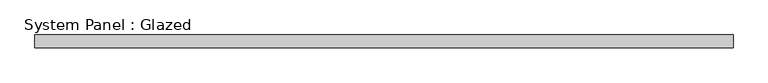
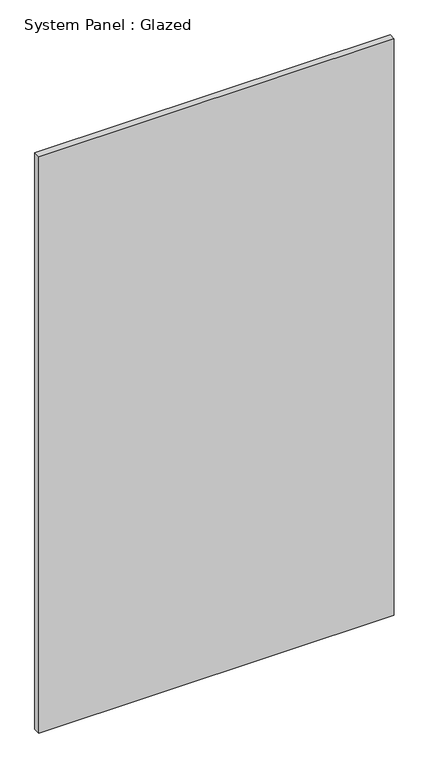
"""IFC4 building model written with IfcOpenShell, lengths in millimetres: plate geometry, System Panel : Glazed."""

from ifc_helpers import new_model, si_unit, origin, origin_with_axes, place, context, project, spatial, polyline, outline, extrude, source, transform, mapped, element, save


def system_panel_glazed_fddb435e(model_context):
    return source(origin(), model_context, "Body", "SweptSolid", [
        extrude(outline(polyline([(683.6833332, 19.05), (-683.6833332, 19.05), (-683.6833332, 44.45), (683.6833332, 44.45), (683.6833332, 19.05)])), origin_with_axes(), (0.0, 0.0, 1.0), 2343.15),
    ])


if __name__ == "__main__":
    model = new_model("IFC4")
    model_context = context("Model", 3, world=origin())
    ifc_project = project(units=[si_unit("LENGTHUNIT", "METRE", prefix="MILLI")], contexts=[model_context])
    site = spatial("IfcSite", under=ifc_project)
    building = spatial("IfcBuilding", under=site)
    placement = place(None, origin())
    system_panel_glazed_shape = system_panel_glazed_fddb435e(model_context)
    element("IfcPlate", 1, ObjectType="System Panel : Glazed", at=placement, inside=building, context=model_context, shape_type="MappedRepresentation", body=[
        mapped(system_panel_glazed_shape, transform((0.0, 0.0, 0.0), x_axis=(1.0, 0.0, 0.0), y_axis=(0.0, 1.0, 0.0), z_axis=(0.0, 0.0, 1.0))),
    ])
    save(model, "model.ifc")

# Revit data of these elements
# Type "System Panel : Glazed"
#   Construction Type Id = "GSP4R"
#   Analytic Construction = "1/8 in Pilkington single glazing"
#   Visual Light Transmittance = 0.9
#   Solar Heat Gain Coefficient = 0.86
#   Heat Transfer Coefficient (U) = 1.18115 BTU/(h·ft²·°F)
#   Define Thermal Properties by = 1
# Element 1 (IfcPlate, "System Panel : Glazed")
#   Materials on its faces: "Glass"
# Materials
#   "Glass": class "Glass", colour RGB 0 128 192, transparency 0.75, Description = "Soda Lime Glass", Cost = 0
